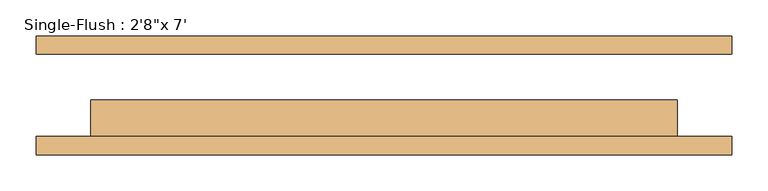
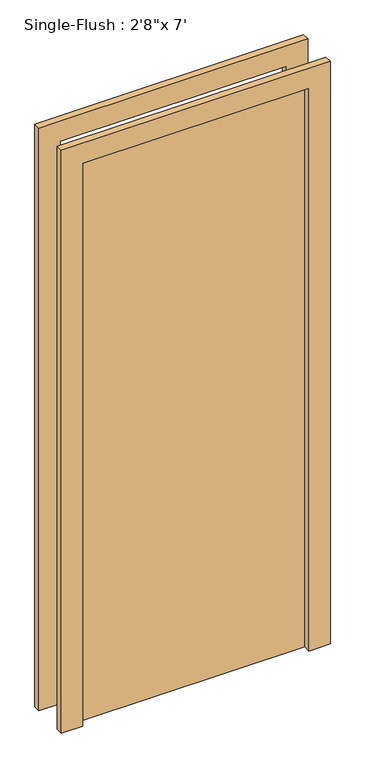
"""IFC4 building model written with IfcOpenShell, lengths in millimetres: door geometry."""

from ifc_helpers import new_model, si_unit, frame, origin, origin_with_axes, place, context, project, spatial, polyline, outline, extrude, source, transform, mapped, element, save


def door_38851409(model_context):
    return source(origin(), model_context, "Body", "SweptSolid", [
        extrude(outline(polyline([(2209.8, -482.6), (0.0, -482.6), (0.0, -406.4), (2133.6, -406.4), (2133.6, 406.4), (0.0, 406.4), (0.0, 482.6), (2209.8, 482.6), (2209.8, -482.6)])), frame((0.0, -82.55, 0.0), z_axis=(0.0, 1.0, 0.0), x_axis=(0.0, 0.0, 1.0)), (0.0, 0.0, 1.0), 25.4),
        extrude(outline(polyline([(2209.8, 482.6), (2209.8, -482.6), (0.0, -482.6), (0.0, -406.4), (2133.6, -406.4), (2133.6, 406.4), (0.0, 406.4), (0.0, 482.6), (2209.8, 482.6)])), frame((0.0, 57.15, 0.0), z_axis=(0.0, 1.0, 0.0), x_axis=(0.0, 0.0, 1.0)), (0.0, 0.0, 1.0), 25.4),
        extrude(outline(polyline([(406.4, -6.35), (406.4, -57.15), (-406.4, -57.15), (-406.4, -6.35), (406.4, -6.35)])), origin_with_axes(), (0.0, 0.0, 1.0), 2133.6),
    ])


if __name__ == "__main__":
    model = new_model("IFC4")
    model_context = context("Model", 3, world=origin())
    ifc_project = project(units=[si_unit("LENGTHUNIT", "METRE", prefix="MILLI")], contexts=[model_context])
    site = spatial("IfcSite", under=ifc_project)
    building = spatial("IfcBuilding", under=site)
    placement = place(None, origin())
    door_shape = door_38851409(model_context)
    element("IfcDoor", 1, ObjectType="Single-Flush : 2'8\"x 7'", at=placement, inside=building, context=model_context, shape_type="MappedRepresentation", body=[
        mapped(door_shape, transform((0.0, 0.0, 0.0), x_axis=(1.0, 0.0, 0.0), y_axis=(0.0, 1.0, 0.0), z_axis=(0.0, 0.0, 1.0))),
    ])
    save(model, "model.ifc")

# Revit data of these elements
# Type "Single-Flush : 2'8\"x 7'"
#   Type Mark = "11"
#   Construction Type Id = "MDOOR"
#   Assembly Code = "C1020"
#   Analytic Construction = "Metal"
#   Thickness = 0' - 2"
#   Heat Transfer Coefficient (U) = 0.651978 BTU/(h·ft²·°F)
#   Height = 7' - 0"
#   Trim Projection Ext = 0' - 1"
#   Trim Projection Int = 0' - 1"
#   Trim Width = 0' - 3"
#   Width = 2' - 8"
#   Define Thermal Properties by = 1
#   Door Material = Door - Panel
#   Frame Material = Door - Frame
#   Visual Light Transmittance = 0
#   Solar Heat Gain Coefficient = 0
#   Function = (empty or 0)
#   Wall Closure = (empty or 0)
# Element 1 (IfcDoor, "Single-Flush : 2'8\"x 7'")
#   Materials on its faces: "Door - Frame", "Door - Panel"
# Materials
#   "Door - Panel": class "Wood", colour RGB 210 159 95, transparency 0, Cost = 0
#   "Door - Frame": colour RGB 118 70 51, transparency 0, Cost = 0
